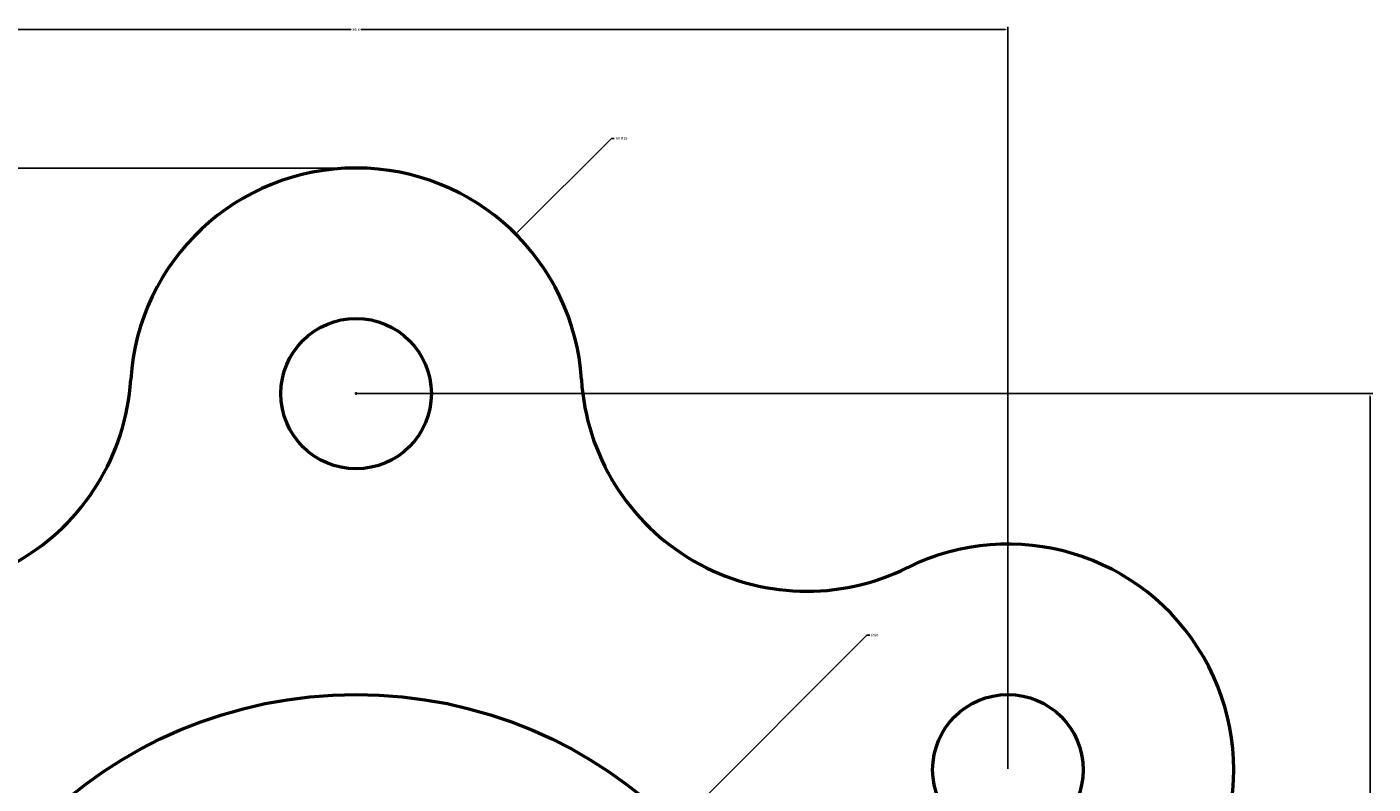
# Model space of a CAD drawing. Units: millimetres. Extents: x 2038 to 2173, y 1596 to 1745.
# Tile 4 of 4: x 2084 to 2173, y 1695 to 1745. Entities that reach past the tile are written whole.
import ezdxf

# ---------------------------------------------------------------- set-up
doc = ezdxf.new("R2010")
doc.units = ezdxf.units.MM
doc.layers.add('M-DIMS', color=2, linetype='Continuous', lineweight=18)
doc.layers.add('M-OUTL', color=7, linetype='Continuous', lineweight=50)
doc.styles.get("Standard").update_dxf_attribs({"font": 'arial.ttf'})
doc.dimstyles.get("Standard").update_dxf_attribs({"dimtxt": 0.18, "dimasz": 0.18, "dimexe": 0.18, "dimexo": 0.0625, "dimgap": 0.09, "dimtad": 0, "dimtih": 1, "dimtoh": 1, "dimdec": 4, "dimzin": 0, "dimdsep": 46, "dimtxsty": 'Standard', "dimcen": 0.09, "dimadec": 0, "dimazin": 0, "dimtfac": 1, "dimtdec": 4, "dimtofl": 0, "dimtmove": 0, "dimatfit": 3, "dimfxl": 1, "dimtolj": 1, "dimtzin": 0, "dimarcsym": 0})

# ---------------------------------------------------------------- blocks, each defined once
blk = doc.blocks.new('*U1')
blk.add_arc((-4.146, 7.965), 15, 243.55731, 356.44269)
blk = doc.blocks.new('*U2')
at = {"layer": 'M-OUTL', "color": 0, "linetype": 'ByBlock', "lineweight": -2, "transparency": 16777216, "rotation": 300}
blk.add_blockref('*U1', (2130.605, 1715.073), dxfattribs=at)
at = {"layer": 'M-OUTL', "color": 0, "linetype": 'ByBlock', "lineweight": -2, "transparency": 16777216}
blk.add_blockref('*U1', (2079.691, 1714.68), dxfattribs=at)
blk = doc.blocks.new('FLANGE-LUG-D10')
blk.add_circle((0, 0), 5)
blk.add_arc((0, 0), 15, 3.55731, 176.44269)
blk = doc.blocks.new('*D5')
at = {"layer": 'Defpoints', "color": 0, "transparency": 16777216}
for p in [(2038.131, 1735.784), (2105.488, 1735.784), (2105.488, 1605.784)]:
    blk.add_point(p, dxfattribs=at)
at = {"layer": 'M-DIMS', "color": 0, "lineweight": -2, "transparency": 16777216}
for p, q in [((2105.425, 1735.784), (2037.951, 1735.784)), ((2038.131, 1735.604), (2038.131, 1670.966)), ((2038.131, 1605.964), (2038.131, 1670.602)), ((2105.425, 1605.784), (2037.951, 1605.784))]:
    blk.add_line(p, q, dxfattribs=at)
at = {"layer": 'M-DIMS', "color": 0, "transparency": 16777216}
for points in [[(2038.101, 1735.604), (2038.161, 1735.604), (2038.131, 1735.784)], [(2038.101, 1605.964), (2038.161, 1605.964), (2038.131, 1605.784)]]:
    blk.add_solid(points, dxfattribs=at)
at = {"layer": 'M-DIMS', "color": 0, "transparency": 16777216, "insert": (2038.131, 1670.784), "char_height": 0.18, "attachment_point": 5}
blk.add_mtext('\\A1;130', dxfattribs=at)
blk = doc.blocks.new('*D6')
at = {"layer": 'Defpoints', "color": 0, "transparency": 16777216}
for p in [(2105.488, 1720.784), (2172.845, 1720.784), (2105.488, 1620.784)]:
    blk.add_point(p, dxfattribs=at)
at = {"layer": 'M-DIMS', "color": 0, "lineweight": -2, "transparency": 16777216}
for p, q in [((2105.55, 1720.784), (2173.025, 1720.784)), ((2172.845, 1720.604), (2172.845, 1670.966)), ((2172.845, 1620.964), (2172.845, 1670.602)), ((2105.55, 1620.784), (2173.025, 1620.784))]:
    blk.add_line(p, q, dxfattribs=at)
at = {"layer": 'M-DIMS', "color": 0, "transparency": 16777216}
for points in [[(2172.815, 1720.604), (2172.875, 1720.604), (2172.845, 1720.784)], [(2172.815, 1620.964), (2172.875, 1620.964), (2172.845, 1620.784)]]:
    blk.add_solid(points, dxfattribs=at)
at = {"layer": 'M-DIMS', "color": 0, "transparency": 16777216, "insert": (2172.845, 1670.784), "char_height": 0.18, "attachment_point": 5}
blk.add_mtext('\\A1;100', dxfattribs=at)
blk = doc.blocks.new('*D8')
at = {"layer": 'Defpoints', "color": 0, "transparency": 16777216}
for p in [(2148.789, 1744.984), (2062.186, 1695.784), (2148.789, 1695.784)]:
    blk.add_point(p, dxfattribs=at)
at = {"layer": 'M-DIMS', "color": 0, "lineweight": -2, "transparency": 16777216}
for p, q in [((2062.186, 1695.847), (2062.186, 1745.164)), ((2062.366, 1744.984), (2105.164, 1744.984)), ((2148.609, 1744.984), (2105.812, 1744.984)), ((2148.789, 1695.847), (2148.789, 1745.164))]:
    blk.add_line(p, q, dxfattribs=at)
at = {"layer": 'M-DIMS', "color": 0, "transparency": 16777216}
for points in [[(2062.366, 1745.014), (2062.366, 1744.954), (2062.186, 1744.984)], [(2148.609, 1745.014), (2148.609, 1744.954), (2148.789, 1744.984)]]:
    blk.add_solid(points, dxfattribs=at)
at = {"layer": 'M-DIMS', "color": 0, "transparency": 16777216, "insert": (2105.488, 1744.984), "char_height": 0.18, "attachment_point": 5}
blk.add_mtext('\\A1;86.6', dxfattribs=at)
blk = doc.blocks.new('*D11')
at = {"layer": 'Defpoints', "color": 0, "transparency": 16777216}
for p in [(2126.701, 1691.998), (2084.275, 1649.571)]:
    blk.add_point(p, dxfattribs=at)
at = {"layer": 'M-DIMS', "color": 0, "lineweight": -2, "transparency": 16777216}
for p, q in [((2139.428, 1704.726), (2126.828, 1692.125)), ((2139.608, 1704.726), (2139.428, 1704.726)), ((2105.398, 1670.784), (2105.578, 1670.784)), ((2105.488, 1670.694), (2105.488, 1670.874))]:
    blk.add_line(p, q, dxfattribs=at)
at = {"layer": 'M-DIMS', "color": 0, "transparency": 16777216}
blk.add_solid([(2126.807, 1692.146), (2126.849, 1692.104), (2126.701, 1691.998)], dxfattribs=at)
at = {"layer": 'M-DIMS', "color": 0, "transparency": 16777216, "insert": (2139.925, 1704.726), "char_height": 0.18, "attachment_point": 5}
blk.add_mtext('\\A1;∅60', dxfattribs=at)
blk = doc.blocks.new('*D12')
at = {"layer": 'Defpoints', "color": 0, "transparency": 16777216}
for p in [(2116.094, 1731.391), (2105.488, 1720.784)]:
    blk.add_point(p, dxfattribs=at)
at = {"layer": 'M-DIMS', "color": 0, "lineweight": -2, "transparency": 16777216}
for p, q in [((2122.458, 1737.755), (2116.221, 1731.518)), ((2122.638, 1737.755), (2122.458, 1737.755)), ((2105.398, 1720.784), (2105.578, 1720.784)), ((2105.488, 1720.694), (2105.488, 1720.874))]:
    blk.add_line(p, q, dxfattribs=at)
at = {"layer": 'M-DIMS', "color": 0, "transparency": 16777216}
blk.add_solid([(2116.2, 1731.54), (2116.243, 1731.497), (2116.094, 1731.391)], dxfattribs=at)
at = {"layer": 'M-DIMS', "color": 0, "transparency": 16777216, "insert": (2123.137, 1737.755), "char_height": 0.18, "attachment_point": 5}
blk.add_mtext('\\A1;6X R15', dxfattribs=at)

msp = doc.modelspace()

# ---------------------------------------------------------------- linework, layer by layer
at = {"layer": 'M-OUTL'}
msp.add_circle((2105.488, 1670.784), 30, dxfattribs=at)

# ---------------------------------------------------------------- block references
for name, p in [('FLANGE-LUG-D10', (2105.488, 1720.784)), ('*U2', (0, 0))]:
    msp.add_blockref(name, p, dxfattribs=at)
at = {"layer": 'M-OUTL', "rotation": 299.9999999999998}
msp.add_blockref('FLANGE-LUG-D10', (2148.789, 1695.784), dxfattribs=at)

# ---------------------------------------------------------------- dimensions: what is measured, and where the dimension line sits
at = {"layer": 'M-DIMS'}
dim = msp.add_linear_dim(base=(2148.789, 1744.984), p1=(2062.186, 1695.784), p2=(2148.789, 1695.784), dimstyle='Standard', override={"dimdec": 1, "dimlfac": 1, "dimrnd": 0, "dimzin": 0, "dimdsep": 46, "dimlunit": 2}, dxfattribs=at)
dim.commit()
dim.dimension.update_dxf_attribs({"geometry": '*D8', "text_midpoint": (2105.488, 1744.984)})
dim = msp.add_radius_dim(center=(2105.488, 1720.784), mpoint=(2116.094, 1731.391), text='6X <>', dimstyle='Standard', override={"dimdec": 0, "dimlfac": 1, "dimrnd": 0, "dimzin": 0, "dimdsep": 46, "dimlunit": 2}, dxfattribs=at)
dim.commit()
dim.dimension.update_dxf_attribs({"geometry": '*D12', "text_midpoint": (2123.137, 1737.755), "dimtype": 164})
for base, p1, p2, picture, middle in [((2038.131, 1735.784), (2105.488, 1605.784), (2105.488, 1735.784), '*D5', (2038.131, 1670.784)), ((2172.845, 1720.784), (2105.488, 1620.784), (2105.488, 1720.784), '*D6', (2172.845, 1670.784))]:
    dim = msp.add_linear_dim(base=base, p1=p1, p2=p2, angle=90, dimstyle='Standard', override={"dimdec": 0, "dimlfac": 1, "dimrnd": 0, "dimzin": 0, "dimdsep": 46, "dimlunit": 2}, dxfattribs=at)
    dim.commit()
    dim.dimension.update_dxf_attribs({"geometry": picture, "text_midpoint": middle})
dim = msp.add_diameter_dim_2p(p1=(2084.275, 1649.571), p2=(2126.701, 1691.998), dimstyle='Standard', override={"dimdec": 0, "dimlfac": 1, "dimrnd": 0, "dimzin": 0, "dimdsep": 46, "dimlunit": 2}, dxfattribs=at)
dim.commit()
dim.dimension.update_dxf_attribs({"geometry": '*D11', "text_midpoint": (2139.925, 1704.726), "dimtype": 163})

doc.saveas('drawing.dxf')
